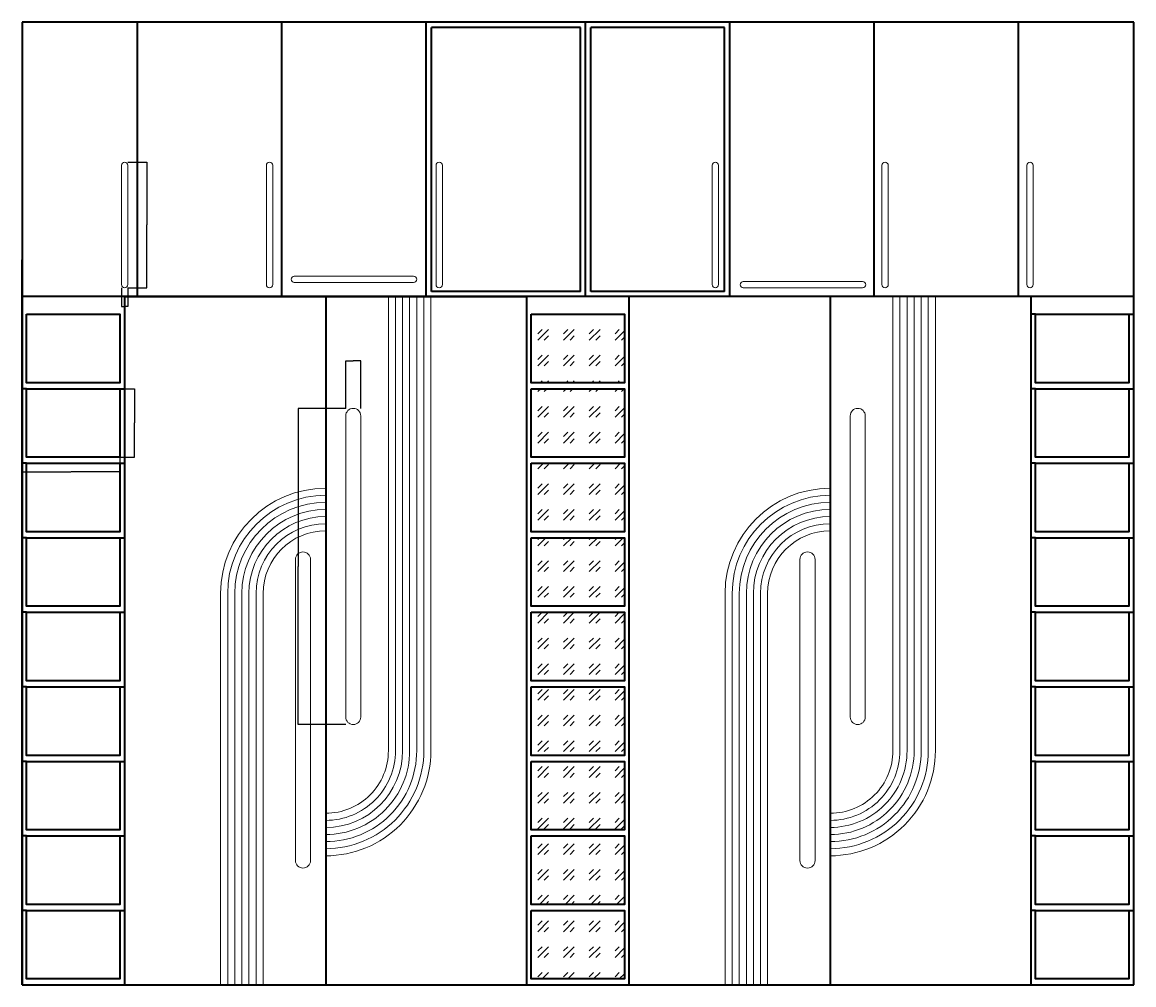
# Model space of a CAD drawing. Units: inches. Extents: x 1252 to 19589, y 1246 to 17124.
import ezdxf

# ---------------------------------------------------------------- set-up
doc = ezdxf.new("R2010")
doc.units = ezdxf.units.IN
doc.header["$MEASUREMENT"] = 0
for name, color, linetype, lineweight in [('A-ANNO-DIMS', 2, 'Continuous', 18), ('A-FURN', 7, 'Continuous', 35), ('A-FURN-DECO', 8, 'Continuous', 18), ('A-FURN-HDWR', 4, 'Continuous', 18), ('A-FURN-PATT', 252, 'Continuous', 13)]:
    doc.layers.add(name, color=color, linetype=linetype, lineweight=lineweight)
doc.styles.get("Standard").update_dxf_attribs({"font": 'arial.ttf'})
doc.dimstyles.get("Standard").update_dxf_attribs({"dimtxt": 0.18, "dimasz": 0.18, "dimexe": 0.18, "dimexo": 0.0625, "dimgap": 0.09, "dimtad": 0, "dimtih": 1, "dimtoh": 1, "dimdec": 4, "dimzin": 0, "dimdsep": 46, "dimtxsty": 'Standard', "dimcen": 0.09, "dimadec": 0, "dimazin": 0, "dimtfac": 1, "dimtdec": 4, "dimtofl": 0, "dimtmove": 0, "dimatfit": 3, "dimfxl": 1, "dimtolj": 1, "dimtzin": 0, "dimarcsym": 0})
pattern_1 = [(45, (0, 0), (424.2640687119285, 0), [250, -350]), (45, (106.066, 0), (424.2640687119285, 0), [100, -500]), (45, (0, 106.066), (424.2640687119285, 0), [100, -500])]

# ---------------------------------------------------------------- blocks, each defined once
blk = doc.blocks.new('SHELF-CUBBY')
blk.add_line((71.39015429980373, 1130.361377618337), (-0.0002032026341112, 1130.361377618337))
blk.add_lwpolyline([(71.39015429980373, 1130.361377618337), (1612.159477089718, 1130.361377618337), (1612.159477089718, -0.0003944745949411), (71.39015429980373, -0.0003944745949411)], close=True)
blk = doc.blocks.new('HANDLE-LOFT')
for points in [[(-0.0001391968662574, 51.988770081849), (-0.0001391968662574, 2020.855460988647)], [(103.9775346902052, 2020.855460988647), (103.9775346902052, 51.988770081849)]]:
    blk.add_lwpolyline(points)
for centre, start, end in [((51.98869774666945, 2020.855460988647), 0, 180), ((51.98869774666945, 51.988770081849), 180, 0)]:
    blk.add_arc(centre, 51.98883694353572, start, end)
blk = doc.blocks.new('HANDLE-PULL')
blk.add_lwpolyline([(248.5541208900895, 124.2769085527566), (248.5541208900895, 5091.690056834539, 0.9999999999999998), (-0.0001924639009303, 5091.690056834539), (-0.0001924639009303, 124.2769085527566)], format="xyb")
blk.add_arc((124.2769642130943, 124.2769085527566), 124.2771566769952, 180, 0)
blk = doc.blocks.new('*D4')
at = {"layer": 'A-ANNO-DIMS', "color": 0, "lineweight": -2, "transparency": 16777216}
for p, q in [((1251.718796797366, 9947.614105525405), (1251.718796797366, 9705.672653481553)), ((2863.878477089718, 9947.614105525405), (2863.878477089718, 9705.672653481553)), ((1251.898796797366, 9705.852653481554), (2056.222838853502, 9705.852653481554)), ((2863.698477089719, 9705.852653481554), (2059.374435033583, 9705.852653481554))]:
    blk.add_line(p, q, dxfattribs=at)
at = {"layer": 'A-ANNO-DIMS', "color": 0, "transparency": 16777216}
for points in [[(1251.898796797366, 9705.882653481553), (1251.898796797366, 9705.822653481551), (1251.718796797366, 9705.852653481554)], [(2863.698477089719, 9705.882653481553), (2863.698477089719, 9705.822653481551), (2863.878477089718, 9705.852653481554)]]:
    blk.add_solid(points, dxfattribs=at)
at = {"layer": 'Defpoints', "color": 0, "transparency": 16777216}
for p in [(1251.718796797366, 9947.676605525405), (2863.878477089718, 9947.676605525405), (2863.878477089718, 9705.852653481554)]:
    blk.add_point(p, dxfattribs=at)
at = {"layer": 'A-ANNO-DIMS', "color": 0, "transparency": 16777216, "insert": (2057.798636943542, 9705.852653481554), "char_height": 0.18, "attachment_point": 5}
blk.add_mtext('\\A1;SHELF CUBBY 1612 TYP.', dxfattribs=at)
blk = doc.blocks.new('*D5')
at = {"layer": 'A-ANNO-DIMS', "color": 0, "lineweight": -2, "transparency": 16777216}
for p, q in [((2863.940977089719, 11078.03837761834), (3105.882429133575, 11078.03837761834)), ((3105.702429133575, 11077.85837761834), (3105.702429133575, 10513.0394561012)), ((3105.702429133575, 9947.856605525409), (3105.702429133575, 10512.67552704254)), ((2863.940977089719, 9947.676605525408), (3105.882429133575, 9947.676605525408))]:
    blk.add_line(p, q, dxfattribs=at)
at = {"layer": 'A-ANNO-DIMS', "color": 0, "transparency": 16777216}
for points in [[(3105.672429133575, 11077.85837761834), (3105.732429133575, 11077.85837761834), (3105.702429133575, 11078.03837761834)], [(3105.672429133575, 9947.856605525409), (3105.732429133575, 9947.856605525409), (3105.702429133575, 9947.676605525408)]]:
    blk.add_solid(points, dxfattribs=at)
at = {"layer": 'Defpoints', "color": 0, "transparency": 16777216}
for p in [(2863.878477089719, 11078.03837761834), (3105.702429133575, 11078.03837761834), (2863.878477089719, 9947.676605525408)]:
    blk.add_point(p, dxfattribs=at)
at = {"layer": 'A-ANNO-DIMS', "color": 0, "transparency": 16777216, "insert": (3105.702429133577, 10512.85749157187), "char_height": 0.18, "attachment_point": 5}
blk.add_mtext('\\A1;1130 TYP.', dxfattribs=at)
blk = doc.blocks.new('*D6')
at = {"layer": 'A-ANNO-DIMS', "color": 0, "lineweight": -2, "transparency": 16777216}
for p, q in [((2994.499034690206, 14815.83829793219), (3305.543189409289, 14815.83829793219)), ((3305.36318940929, 14815.65829793219), (3305.36318940929, 13779.59930789542)), ((3305.36318940929, 12743.17393313832), (3305.36318940929, 13779.23292317509)), ((2994.499034690206, 12742.99393313832), (3305.54318940929, 12742.99393313832))]:
    blk.add_line(p, q, dxfattribs=at)
at = {"layer": 'A-ANNO-DIMS', "color": 0, "transparency": 16777216}
for points in [[(3305.333189409289, 14815.65829793219), (3305.393189409289, 14815.65829793219), (3305.36318940929, 14815.83829793219)], [(3305.333189409289, 12743.17393313832), (3305.39318940929, 12743.17393313832), (3305.36318940929, 12742.99393313832)]]:
    blk.add_solid(points, dxfattribs=at)
at = {"layer": 'Defpoints', "color": 0, "transparency": 16777216}
for p in [(2994.436534690206, 14815.83829793219), (3305.36318940929, 14815.83829793219), (2994.436534690206, 12742.99393313832)]:
    blk.add_point(p, dxfattribs=at)
at = {"layer": 'A-ANNO-DIMS', "color": 0, "transparency": 16777216, "insert": (3305.363189409292, 13779.41611553525), "char_height": 0.18, "attachment_point": 5}
blk.add_mtext('\\A1;LOFT HANDLE 2073 TYP.', dxfattribs=at)
blk = doc.blocks.new('*D7')
at = {"layer": 'A-ANNO-DIMS', "color": 0, "lineweight": -2, "transparency": 16777216}
for p, q in [((2890.458860803134, 12742.93143313831), (2890.458860803134, 12431.88727841923)), ((2994.436534690205, 12742.93143313831), (2994.436534690205, 12431.88727841923)), ((2890.638860803134, 12432.06727841923), (2941.858154772591, 12432.06727841923)), ((2994.256534690205, 12432.06727841923), (2943.037240720748, 12432.06727841923))]:
    blk.add_line(p, q, dxfattribs=at)
at = {"layer": 'A-ANNO-DIMS', "color": 0, "transparency": 16777216}
for points in [[(2890.638860803134, 12432.09727841923), (2890.638860803134, 12432.03727841923), (2890.458860803134, 12432.06727841923)], [(2994.256534690205, 12432.09727841923), (2994.256534690205, 12432.03727841923), (2994.436534690205, 12432.06727841923)]]:
    blk.add_solid(points, dxfattribs=at)
at = {"layer": 'Defpoints', "color": 0, "transparency": 16777216}
for p in [(2890.458860803134, 12742.99393313831), (2994.436534690205, 12742.99393313831), (2994.436534690205, 12432.06727841923)]:
    blk.add_point(p, dxfattribs=at)
at = {"layer": 'A-ANNO-DIMS', "color": 0, "transparency": 16777216, "insert": (2942.447697746669, 12432.06727841923), "char_height": 0.18, "attachment_point": 5}
blk.add_mtext('\\A1;104 TYP.', dxfattribs=at)
blk = doc.blocks.new('*D8')
at = {"layer": 'A-ANNO-DIMS', "color": 0, "lineweight": -2, "transparency": 16777216}
for p, q in [((6588.23961462363, 10754.15993410268), (5805.726995378264, 10754.15993410268)), ((5805.906995378264, 10753.97993410267), (5805.906995378265, 8146.359334253412)), ((5805.906995378265, 5538.372472466903), (5805.906995378265, 8145.993072316167)), ((6588.23961462363, 5538.192472466903), (5805.726995378265, 5538.192472466903))]:
    blk.add_line(p, q, dxfattribs=at)
at = {"layer": 'A-ANNO-DIMS', "color": 0, "transparency": 16777216}
for points in [[(5805.876995378264, 10753.97993410267), (5805.936995378264, 10753.97993410267), (5805.906995378264, 10754.15993410268)], [(5805.876995378266, 5538.372472466903), (5805.936995378266, 5538.372472466903), (5805.906995378265, 5538.192472466903)]]:
    blk.add_solid(points, dxfattribs=at)
at = {"layer": 'Defpoints', "color": 0, "transparency": 16777216}
for p in [(5805.906995378264, 10754.15993410268), (6588.30211462363, 10754.15993410268), (6588.30211462363, 5538.192472466903)]:
    blk.add_point(p, dxfattribs=at)
at = {"layer": 'A-ANNO-DIMS', "color": 0, "transparency": 16777216, "insert": (5805.906995378267, 8146.176203284786), "char_height": 0.18, "attachment_point": 5}
blk.add_mtext('\\A1;DOOR PULL HANDLE 5216 TYP.', dxfattribs=at)
blk = doc.blocks.new('*D9')
at = {"layer": 'A-ANNO-DIMS', "color": 0, "lineweight": -2, "transparency": 16777216}
for p, q in [((6588.302114623627, 10754.22243410267), (6588.302114623627, 11536.73505334804)), ((6588.482114623627, 11536.55505334804), (6711.97972150526, 11536.55505334804)), ((6836.676427977618, 11536.55505334804), (6713.178821095984, 11536.55505334804)), ((6836.856427977618, 10754.22243410267), (6836.856427977618, 11536.73505334804))]:
    blk.add_line(p, q, dxfattribs=at)
at = {"layer": 'A-ANNO-DIMS', "color": 0, "transparency": 16777216}
for points in [[(6588.482114623627, 11536.58505334804), (6588.482114623627, 11536.52505334804), (6588.302114623627, 11536.55505334804)], [(6836.676427977618, 11536.58505334804), (6836.676427977618, 11536.52505334804), (6836.856427977618, 11536.55505334804)]]:
    blk.add_solid(points, dxfattribs=at)
at = {"layer": 'Defpoints', "color": 0, "transparency": 16777216}
for p in [(6836.856427977618, 11536.55505334804), (6588.302114623627, 10754.15993410267), (6836.856427977618, 10754.15993410267)]:
    blk.add_point(p, dxfattribs=at)
at = {"layer": 'A-ANNO-DIMS', "color": 0, "transparency": 16777216, "insert": (6712.579271300622, 11536.55505334804), "char_height": 0.18, "attachment_point": 5}
blk.add_mtext('\\A1;249 TYP.', dxfattribs=at)

msp = doc.modelspace()

# ---------------------------------------------------------------- hatches: boundary and pattern name
at = {"layer": 'A-FURN-PATT'}
h = msp.add_hatch(dxfattribs=at)
h.set_pattern_fill('GOST_GLASS', color=256, scale=50)
h.set_pattern_definition(pattern_1)
h.paths.add_polyline_path([(11186.71865364294, 12307.49529997785), (9645.94933085303, 12307.49529997785), (9645.94933085303, 11177.13352788492), (11186.71865364294, 11177.13352788492)])
h = msp.add_hatch(dxfattribs=at)
h.set_pattern_fill('GOST_GLASS', color=256, scale=50)
h.set_pattern_definition(pattern_1)
h.paths.add_polyline_path([(11186.71865364294, 11078.03837761833), (9645.94933085303, 11078.03837761833), (9645.94933085303, 9947.676605525405), (11186.71865364294, 9947.676605525405)])
h.paths.add_polyline_path([(11186.71865364294, 9848.58145525882), (9645.94933085303, 9848.58145525882), (9645.94933085303, 8718.219683165888), (11186.71865364294, 8718.219683165888)])
h.paths.add_polyline_path([(11186.71865364294, 8619.124532899305), (9645.94933085303, 8619.124532899305), (9645.94933085303, 7488.762760806371), (11186.71865364294, 7488.762760806371)])
h.paths.add_polyline_path([(11186.71865364294, 7389.667610539786), (9645.94933085303, 7389.667610539786), (9645.94933085303, 6259.305838446853), (11186.71865364294, 6259.305838446853)])
h.paths.add_polyline_path([(11186.71865364294, 6160.210688180269), (9645.94933085303, 6160.210688180268), (9645.94933085303, 5029.848916087336), (11186.71865364294, 5029.848916087336)])
h.paths.add_polyline_path([(11186.71865364294, 4930.753765820751), (9645.94933085303, 4930.753765820751), (9645.94933085303, 3800.39199372782), (11186.71865364294, 3800.39199372782)])
h.paths.add_polyline_path([(11186.71865364294, 3701.296843461234), (9645.94933085303, 3701.296843461234), (9645.94933085303, 2570.935071368302), (11186.71865364294, 2570.935071368302)])
h.paths.add_polyline_path([(11186.71865364294, 2471.839921101716), (9645.94933085303, 2471.839921101716), (9645.94933085303, 1341.478149008786), (11186.71865364294, 1341.478149008784)])

# ---------------------------------------------------------------- linework, layer by layer
at = {"layer": 'A-FURN'}
for p, q in [((19588.89400300624, 17123.61266904812), (1251.718796797366, 17123.61266904812)), ((1251.718796797366, 17123.61266904812), (1251.718796797366, 1245.72494442021)), ((3153.26554302359, 12596.97935484337), (3153.265543023591, 17123.61266904812)), ((5533.517518042849, 12596.97935484337), (5533.517518042849, 17123.61266904812)), ((7913.769493062108, 12596.97935484337), (7913.769493062108, 17123.61266904812)), ((10546.59133172224, 12596.97935484337), (10546.59133172224, 17123.61266904812)), ((12926.8433067415, 12596.97935484337), (12926.8433067415, 17123.61266904812)), ((15307.09528176076, 12596.97935484337), (15307.09528176076, 17123.61266904812)), ((17687.34725678002, 12596.97935484337), (17687.34725678002, 17123.61266904812)), ((19588.89400300624, 1245.72494442021), (19588.89400300624, 17123.61266904812)), ((8000.975276084281, 12684.18513786554), (8000.975276084281, 17036.40688602595)), ((10459.38554870007, 17036.40688602595), (8000.975276084279, 17036.40688602595)), ((10459.38554870007, 12684.18513786554), (10459.38554870007, 17036.40688602595)), ((10633.79711474441, 12684.18513786554), (10633.79711474441, 17036.40688602595)), ((12839.63752371933, 17036.40688602594), (10633.79711474441, 17036.40688602595)), ((12839.63752371933, 12684.18513786554), (12839.63752371933, 17036.40688602595)), ((1251.718796797366, 1245.72494442021), (1251.718796797366, 13201.74396838631)), ((19588.89400300624, 1245.72494442021), (19588.89400300624, 13201.74396838631)), ((10459.38554870007, 12684.18513786554), (8000.975276084281, 12684.18513786554)), ((12839.63752371933, 12684.18513786554), (10633.79711474441, 12684.18513786554)), ((19588.89400300624, 12596.97935484337), (1251.718796797366, 12596.97935484337)), ((2943.213649899794, 1245.72494442021), (2943.213649899794, 12596.97935484337)), ((2943.213649899794, 12596.97935484337), (9574.55897335059, 12596.97935484337)), ((6258.886311625192, 12596.97935484337), (6258.886311625192, 8734.854201615286)), ((9574.55897335059, 1245.72494442021), (9574.55897335059, 12596.97935484337)), ((11266.05382645302, 1245.72494442021), (11266.05382645302, 12596.97935484337)), ((14581.72648817842, 12596.97935484337), (14581.72648817841, 1245.72494442021)), ((14581.72648817842, 12596.97935484337), (14581.72648817842, 8734.854201615286)), ((17897.39914990381, 1245.72494442021), (17897.39914990382, 12596.97935484337)), ((19509.55883019617, 12307.49529997785), (19588.89400300624, 12307.49529997785)), ((2863.878477089718, 11078.03837761833), (2943.213649899793, 11078.03837761833)), ((19509.55883019617, 11078.03837761833), (19588.89400300624, 11078.03837761833)), ((2863.878477089718, 9848.58145525882), (2943.213649899793, 9848.581455258818)), ((19509.55883019617, 9848.58145525882), (19588.89400300624, 9848.58145525882)), ((2863.878477089718, 8619.124532899305), (2943.213649899793, 8619.124532899305)), ((6258.886311625193, 8734.854201615286), (6258.886311625191, 4074.471821968992)), ((14581.72648817842, 8734.854201615286), (14581.72648817842, 4074.471821968992)), ((19509.55883019617, 8619.124532899305), (19588.89400300624, 8619.124532899305)), ((2863.878477089718, 7389.667610539786), (2943.213649899793, 7389.667610539785)), ((19509.55883019617, 7389.667610539786), (19588.89400300624, 7389.667610539786)), ((2863.878477089718, 6160.210688180268), (2943.213649899793, 6160.210688180267)), ((19509.55883019617, 6160.210688180268), (19588.89400300624, 6160.210688180268)), ((2863.878477089718, 4930.753765820751), (2943.213649899793, 4930.753765820751)), ((19509.55883019617, 4930.753765820751), (19588.89400300624, 4930.753765820751)), ((6258.886311625191, 4074.471821968992), (6258.886311625191, 1245.72494442021)), ((14581.72648817842, 4074.471821968992), (14581.72648817842, 1245.72494442021)), ((2863.878477089718, 3701.296843461234), (2943.213649899793, 3701.296843461234)), ((19509.55883019617, 3701.296843461234), (19588.89400300624, 3701.296843461234)), ((2863.878477089718, 2471.839921101717), (2943.213649899793, 2471.839921101717)), ((19509.55883019617, 2471.839921101717), (19588.89400300624, 2471.839921101717)), ((1251.718796797366, 1245.72494442021), (19588.89400300624, 1245.72494442021))]:
    msp.add_line(p, q, dxfattribs=at)
for points in [[(1323.109154299804, 12307.49529997785), (2863.878477089718, 12307.49529997785), (2863.878477089718, 11177.13352788492), (1323.109154299804, 11177.13352788492)], [(9645.94933085303, 12307.49529997785), (11186.71865364294, 12307.49529997785), (11186.71865364294, 11177.13352788492), (9645.94933085303, 11177.13352788492)], [(9645.94933085303, 11078.03837761833), (11186.71865364294, 11078.03837761833), (11186.71865364294, 9947.676605525405), (9645.94933085303, 9947.676605525405)], [(9645.94933085303, 9848.58145525882), (11186.71865364294, 9848.58145525882), (11186.71865364294, 8718.219683165888), (9645.94933085303, 8718.219683165888)], [(9645.94933085303, 8619.124532899305), (11186.71865364294, 8619.124532899305), (11186.71865364294, 7488.762760806371), (9645.94933085303, 7488.762760806371)], [(9645.94933085303, 7389.667610539786), (11186.71865364294, 7389.667610539786), (11186.71865364294, 6259.305838446853), (9645.94933085303, 6259.305838446853)], [(9645.94933085303, 6160.210688180268), (11186.71865364294, 6160.210688180268), (11186.71865364294, 5029.848916087336), (9645.94933085303, 5029.848916087336)], [(9645.94933085303, 4930.753765820751), (11186.71865364294, 4930.753765820751), (11186.71865364294, 3800.391993727819), (9645.94933085303, 3800.391993727819)], [(9645.94933085303, 3701.296843461234), (11186.71865364294, 3701.296843461234), (11186.71865364294, 2570.935071368302), (9645.94933085303, 2570.935071368302)], [(9645.94933085303, 2471.839921101717), (11186.71865364294, 2471.839921101717), (11186.71865364294, 1341.478149008784), (9645.94933085303, 1341.478149008784)]]:
    msp.add_lwpolyline(points, close=True, dxfattribs=at)
at = {"layer": 'A-FURN-DECO'}
for p, q in [((4523.894798499845, 7701.475925935982), (4523.894798499845, 1245.72494442021)), ((4640.830338074185, 7701.475925935982), (4640.830338074185, 1245.72494442021)), ((4757.765877648526, 7701.475925935982), (4757.765877648526, 1245.72494442021)), ((4874.701417222866, 7701.475925935982), (4874.701417222866, 1245.72494442021)), ((4991.636956797207, 7701.475925935982), (4991.636956797207, 1245.72494442021)), ((5108.572496371547, 7701.475925935982), (5108.572496371547, 1245.72494442021)), ((5225.508035945888, 7701.475925935982), (5225.508035945888, 1245.72494442021)), ((12846.73497505307, 7701.475925935982), (12846.73497505307, 1245.72494442021)), ((12963.67051462741, 7701.475925935982), (12963.67051462741, 1245.72494442021)), ((13080.60605420175, 7701.475925935982), (13080.60605420175, 1245.72494442021)), ((13197.54159377609, 7701.475925935982), (13197.54159377609, 1245.72494442021)), ((13314.47713335043, 7701.475925935982), (13314.47713335043, 1245.72494442021)), ((13431.41267292477, 7701.475925935982), (13431.41267292477, 1245.72494442021)), ((13548.34821249911, 7701.475925935982), (13548.34821249911, 1245.72494442021))]:
    msp.add_line(p, q, dxfattribs=at)
for points in [[(6258.886311625191, 4074.471821968992, 0.4142135623730951), (7292.264587304497, 5107.850097648298), (7292.264587304497, 12596.97935484337)], [(6258.886311625191, 3957.536282394652, 0.4142135623730951), (7409.200126878838, 5107.850097648298), (7409.200126878838, 12596.97935484337)], [(6258.886311625191, 3840.600742820311, 0.4142135623730951), (7526.135666453177, 5107.850097648298), (7526.135666453178, 12596.97935484337)], [(6258.886311625191, 3723.665203245971, 0.4142135623730951), (7643.071206027518, 5107.850097648298), (7643.07120602752, 12596.97935484337)], [(6258.886311625191, 3606.72966367163, 0.4142135623730951), (7760.006745601859, 5107.850097648298), (7760.006745601859, 12596.97935484337)], [(6258.886311625191, 3489.79412409729, 0.4142135623730951), (7876.942285176198, 5107.850097648298), (7876.9422851762, 12596.97935484337)], [(6258.886311625191, 3372.858584522949, 0.4142135623730951), (7993.87782475054, 5107.850097648298), (7993.877824750541, 12596.97935484337)], [(14581.72648817842, 4074.471821968992, 0.4142135623730951), (15615.10476385772, 5107.850097648298), (15615.10476385772, 12596.97935484337)], [(14581.72648817842, 3957.536282394652, 0.4142135623730951), (15732.04030343206, 5107.850097648298), (15732.04030343206, 12596.97935484337)], [(14581.72648817842, 3840.600742820311, 0.4142135623730951), (15848.9758430064, 5107.850097648298), (15848.9758430064, 12596.97935484337)], [(14581.72648817842, 3723.665203245971, 0.4142135623730951), (15965.91138258074, 5107.850097648298), (15965.91138258074, 12596.97935484337)], [(14581.72648817842, 3606.72966367163, 0.4142135623730951), (16082.84692215508, 5107.850097648298), (16082.84692215508, 12596.97935484337)], [(14581.72648817842, 3489.79412409729, 0.4142135623730951), (16199.78246172942, 5107.850097648298), (16199.78246172942, 12596.97935484337)], [(14581.72648817842, 3372.858584522949, 0.4142135623730951), (16316.71800130376, 5107.850097648298), (16316.71800130376, 12596.97935484337)]]:
    msp.add_lwpolyline(points, format="xyb", dxfattribs=at)
for centre, radius, start in [((6258.886311625193, 7701.475925935982), 1734.991513125348, 90.00000000000003), ((14581.72648817842, 7701.475925935982), 1734.991513125348, 90), ((6258.886311625193, 7701.475925935982), 1618.055973551008, 90.00000000000003), ((6258.886311625193, 7701.475925935982), 1501.120433976667, 90.00000000000003), ((14581.72648817842, 7701.475925935982), 1618.055973551008, 90), ((14581.72648817842, 7701.475925935982), 1501.120433976667, 90), ((6258.886311625193, 7701.475925935982), 1384.184894402327, 90.00000000000003), ((14581.72648817842, 7701.475925935982), 1384.184894402327, 90), ((6258.886311625193, 7701.475925935982), 1267.249354827986, 90.00000000000003), ((6258.886311625193, 7701.475925935982), 1150.313815253646, 90.00000000000003), ((14581.72648817842, 7701.475925935982), 1267.249354827986, 90), ((14581.72648817842, 7701.475925935982), 1150.313815253646, 90), ((6258.886311625193, 7701.475925935982), 1033.378275679305, 90.00000000000003), ((14581.72648817842, 7701.475925935982), 1033.378275679305, 90)]:
    msp.add_arc(centre, radius, start, 180, dxfattribs=at)

# ---------------------------------------------------------------- block references
at = {"layer": 'A-FURN'}
for p in [(17897.39935310645, 11177.13392235952), (1251.719, 9947.677), (17897.39935310645, 9947.677), (1251.718999999997, 8718.220077640492), (17897.39935310645, 8718.22007764049), (1251.718999999997, 7488.763155280975), (17897.39935310645, 7488.763155280975), (1251.718999999998, 6259.306232921455), (17897.39935310645, 6259.306232921455), (1251.718999999997, 5029.849310561939), (17897.39935310644, 5029.849310561939), (1251.718999999997, 3800.392388202422), (17897.39935310645, 3800.392388202422), (1251.718999999998, 2570.935465842904), (17897.39935310645, 2570.935465842904), (1251.718999999997, 1341.478543483386), (17897.39935310644, 1341.478543483386)]:
    msp.add_blockref('SHELF-CUBBY', p, dxfattribs=at)
at = {"layer": 'A-FURN-HDWR'}
for name, p in [('HANDLE-LOFT', (2890.459, 12742.994)), ('HANDLE-LOFT', (5279.302647433415, 12742.994)), ('HANDLE-LOFT', (8078.771983100883, 12742.994)), ('HANDLE-LOFT', (12634.556264646, 12742.994)), ('HANDLE-LOFT', (15434.62009919859, 12742.994)), ('HANDLE-LOFT', (17826.15773079951, 12742.994)), ('HANDLE-PULL', (6588.302307087528, 5538.19272059114)), ('HANDLE-PULL', (14911.14248364075, 5538.19272059114)), ('HANDLE-PULL', (5759.046999999999, 3170.065)), ('HANDLE-PULL', (14081.88717655322, 3170.065000000001))]:
    msp.add_blockref(name, p, dxfattribs=at)
for p, rotation in [((5687.153782905225, 12935.93112137138), 269.9999999999997), ((13095.05141189316, 12845.17418727563), 270)]:
    msp.add_blockref('HANDLE-LOFT', p, dxfattribs=dict(at, rotation=rotation))

# ---------------------------------------------------------------- dimensions: what is measured, and where the dimension line sits
at = {"layer": 'A-ANNO-DIMS'}
for base, p1, p2, text, picture, middle in [((3305.36318940929, 14815.83829793219), (2994.436534690205, 12742.99393313831), (2994.436534690205, 14815.83829793218), 'LOFT HANDLE <> TYP.', '*D6', (3305.363189409292, 13779.41611553525)), ((3105.702429133575, 11078.03837761834), (2863.878477089718, 9947.676605525405), (2863.878477089718, 11078.03837761833), '<> TYP.', '*D5', (3105.702429133577, 10512.85749157187)), ((5805.906995378264, 10754.15993410268), (6588.302114623627, 5538.192472466902), (6588.302114623627, 10754.15993410267), 'DOOR PULL HANDLE <> TYP.', '*D8', (5805.906995378267, 8146.176203284786))]:
    dim = msp.add_linear_dim(base=base, p1=p1, p2=p2, angle=90, text=text, dimstyle='Standard', override={"dimdec": 0, "dimlfac": 1, "dimrnd": 0, "dimzin": 0, "dimdsep": 46, "dimlunit": 2}, dxfattribs=at)
    dim.commit()
    dim.dimension.update_dxf_attribs({"geometry": picture, "text_midpoint": middle})
for base, p1, p2, text, picture, middle in [((2994.436534690205, 12432.06727841923), (2890.458860803134, 12742.99393313831), (2994.436534690205, 12742.99393313831), '<> TYP.', '*D7', (2942.447697746669, 12432.06727841923)), ((6836.856427977618, 11536.55505334804), (6588.302114623627, 10754.15993410267), (6836.856427977618, 10754.15993410267), '<> TYP.', '*D9', (6712.579271300622, 11536.55505334804)), ((2863.878477089718, 9705.852653481554), (1251.718796797366, 9947.676605525405), (2863.878477089718, 9947.676605525405), 'SHELF CUBBY <> TYP.', '*D4', (2057.798636943542, 9705.852653481554))]:
    dim = msp.add_linear_dim(base=base, p1=p1, p2=p2, text=text, dimstyle='Standard', override={"dimdec": 0, "dimlfac": 1, "dimrnd": 0, "dimzin": 0, "dimdsep": 46, "dimlunit": 2}, dxfattribs=at)
    dim.commit()
    dim.dimension.update_dxf_attribs({"geometry": picture, "text_midpoint": middle})

doc.saveas('drawing.dxf')
